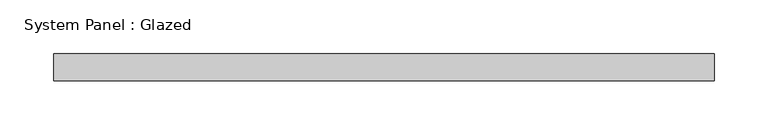
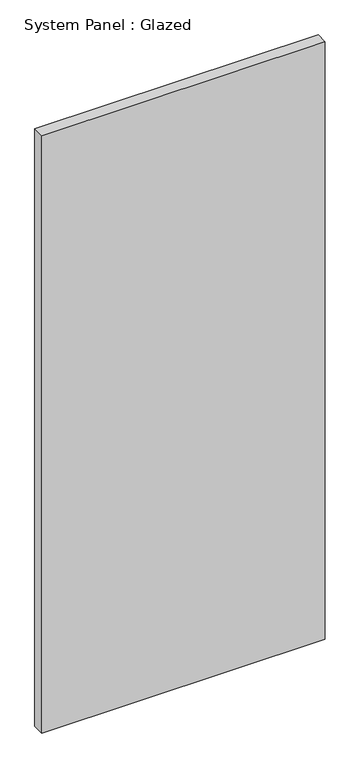
"""IFC4 building model written with IfcOpenShell, lengths in millimetres: plate geometry, System Panel : Glazed."""

from ifc_helpers import new_model, si_unit, origin, origin_with_axes, place, context, project, spatial, polyline, outline, extrude, source, transform, mapped, element, save


def system_panel_glazed_7001ef1f(model_context):
    return source(origin(), model_context, "Body", "SweptSolid", [
        extrude(outline(polyline([(307.975, 19.05), (-307.975, 19.05), (-307.975, 44.45), (307.975, 44.45), (307.975, 19.05)])), origin_with_axes(), (0.0, 0.0, 1.0), 1371.695751),
    ])


if __name__ == "__main__":
    model = new_model("IFC4")
    model_context = context("Model", 3, world=origin())
    ifc_project = project(units=[si_unit("LENGTHUNIT", "METRE", prefix="MILLI")], contexts=[model_context])
    site = spatial("IfcSite", under=ifc_project)
    building = spatial("IfcBuilding", under=site)
    placement = place(None, origin())
    system_panel_glazed_shape = system_panel_glazed_7001ef1f(model_context)
    element("IfcPlate", 1, ObjectType="System Panel : Glazed", at=placement, inside=building, context=model_context, shape_type="MappedRepresentation", body=[
        mapped(system_panel_glazed_shape, transform((0.0, 0.0, 0.0), x_axis=(1.0, 0.0, 0.0), y_axis=(0.0, 1.0, 0.0), z_axis=(0.0, 0.0, 1.0))),
    ])
    save(model, "model.ifc")

# Revit data of these elements
# Type "System Panel : Glazed"
#   Construction Type Id = "GSP4R"
#   Analytic Construction = "1/8 in Pilkington single glazing"
#   Visual Light Transmittance = 0.9
#   Solar Heat Gain Coefficient = 0.86
#   Heat Transfer Coefficient (U) = 1.18115 BTU/(h·ft²·°F)
#   Define Thermal Properties by = 1
# Element 1 (IfcPlate, "System Panel : Glazed")
#   Materials on its faces: "Glass"
# Materials
#   "Glass": class "Glass", colour RGB 0 128 192, transparency 0.75, Description = "Soda Lime Glass", Cost = 0
